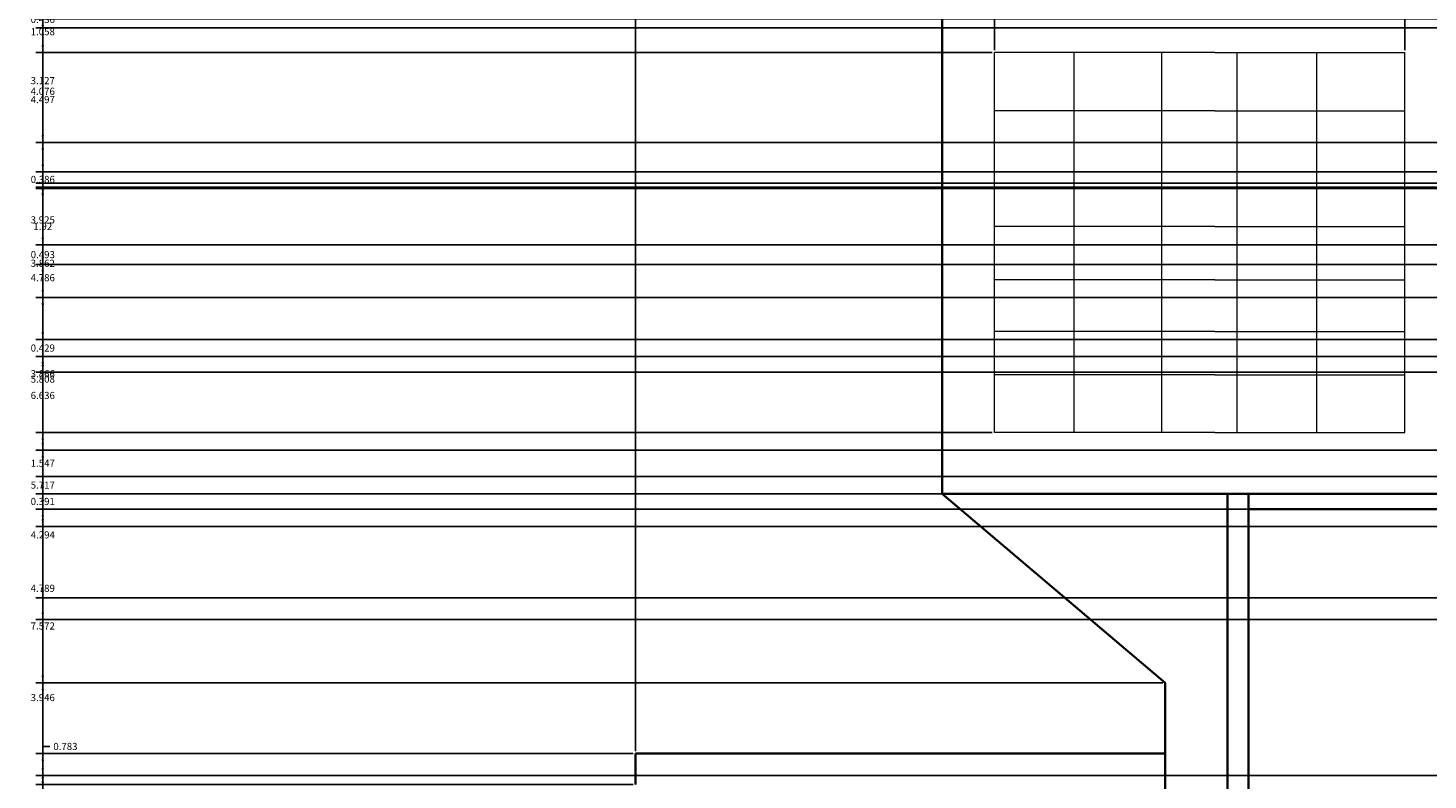
# Model space of a CAD drawing. Units: inches. Extents: x -10 to 130, y -32 to 34.
# Tile 2 of 22: x -10 to 26, y -13 to 6. Entities that reach past the tile are written whole.
import ezdxf

# ---------------------------------------------------------------- set-up
doc = ezdxf.new("R2010")
doc.units = ezdxf.units.IN
doc.header["$MEASUREMENT"] = 0
for name, color, linetype, lineweight in [('A-ANNO-DIMS', 2, 'Continuous', 18), ('A-ELEV', 7, 'Continuous', 35), ('A-GLAZ', 4, 'Continuous', 18)]:
    doc.layers.add(name, color=color, linetype=linetype, lineweight=lineweight)
doc.styles.get("Standard").update_dxf_attribs({"font": 'arial.ttf'})
doc.dimstyles.get("Standard").update_dxf_attribs({"dimtxt": 0.18, "dimasz": 0.18, "dimexe": 0.18, "dimexo": 0.0625, "dimgap": 0.09, "dimtad": 0, "dimtih": 1, "dimtoh": 1, "dimdec": 4, "dimzin": 0, "dimdsep": 46, "dimtxsty": 'Standard', "dimcen": 0.09, "dimadec": 0, "dimazin": 0, "dimtfac": 1, "dimtdec": 4, "dimtofl": 0, "dimtmove": 0, "dimatfit": 3, "dimfxl": 1, "dimtolj": 1, "dimtzin": 0, "dimarcsym": 0})

# ---------------------------------------------------------------- blocks, each defined once
blk = doc.blocks.new('*D11')
at = {"layer": 'A-ANNO-DIMS', "color": 0, "lineweight": -2, "transparency": 16777216}
for p, q in [((5.634, -12.739), (5.634, 33.879)), ((19.588, 19.547), (19.588, 33.879)), ((5.814, 33.699), (12.156, 33.699)), ((19.408, 33.699), (13.066, 33.699))]:
    blk.add_line(p, q, dxfattribs=at)
at = {"layer": 'A-ANNO-DIMS', "color": 0, "transparency": 16777216}
for points in [[(5.814, 33.729), (5.814, 33.669), (5.634, 33.699)], [(19.408, 33.729), (19.408, 33.669), (19.588, 33.699)]]:
    blk.add_solid(points, dxfattribs=at)
at = {"layer": 'Defpoints', "color": 0, "transparency": 16777216}
for p in [(19.588, 33.699), (19.588, 19.485), (5.634, -12.801)]:
    blk.add_point(p, dxfattribs=at)
at = {"layer": 'A-ANNO-DIMS', "color": 0, "transparency": 16777216, "insert": (12.611, 33.699), "char_height": 0.18, "attachment_point": 5}
blk.add_mtext('\\A1;13.954', dxfattribs=at)
blk = doc.blocks.new('*D30')
at = {"layer": 'A-ANNO-DIMS', "color": 0, "lineweight": -2, "transparency": 16777216}
for p, q in [((18.993, -11.011), (-9.564, -11.011)), ((-9.384, -11.191), (-9.384, -16.031)), ((-9.384, -21.234), (-9.384, -16.394)), ((8.226, -21.414), (-9.564, -21.414))]:
    blk.add_line(p, q, dxfattribs=at)
at = {"layer": 'A-ANNO-DIMS', "color": 0, "transparency": 16777216}
for points in [[(-9.414, -11.191), (-9.354, -11.191), (-9.384, -11.011)], [(-9.414, -21.234), (-9.354, -21.234), (-9.384, -21.414)]]:
    blk.add_solid(points, dxfattribs=at)
at = {"layer": 'Defpoints', "color": 0, "transparency": 16777216}
for p in [(-9.384, -11.011), (19.055, -11.011), (8.289, -21.414)]:
    blk.add_point(p, dxfattribs=at)
at = {"layer": 'A-ANNO-DIMS', "color": 0, "transparency": 16777216, "insert": (-9.384, -16.213), "char_height": 0.18, "attachment_point": 5}
blk.add_mtext('\\A1;10.404', dxfattribs=at)
blk = doc.blocks.new('*D31')
at = {"layer": 'A-ANNO-DIMS', "color": 0, "lineweight": -2, "transparency": 16777216}
for p, q in [((13.34, -6.222), (-9.564, -6.222)), ((-9.384, -6.402), (-9.384, -8.434)), ((-9.384, -10.831), (-9.384, -8.798)), ((18.993, -11.011), (-9.564, -11.011))]:
    blk.add_line(p, q, dxfattribs=at)
at = {"layer": 'A-ANNO-DIMS', "color": 0, "transparency": 16777216}
for points in [[(-9.414, -6.402), (-9.354, -6.402), (-9.384, -6.222)], [(-9.414, -10.831), (-9.354, -10.831), (-9.384, -11.011)]]:
    blk.add_solid(points, dxfattribs=at)
at = {"layer": 'Defpoints', "color": 0, "transparency": 16777216}
for p in [(-9.384, -6.222), (13.402, -6.222), (19.055, -11.011)]:
    blk.add_point(p, dxfattribs=at)
at = {"layer": 'A-ANNO-DIMS', "color": 0, "transparency": 16777216, "insert": (-9.384, -8.616), "char_height": 0.18, "attachment_point": 5}
blk.add_mtext('\\A1;4.789', dxfattribs=at)
blk = doc.blocks.new('*D32')
at = {"layer": 'A-ANNO-DIMS', "color": 0, "lineweight": -2, "transparency": 16777216}
for p, q in [((31.909, -0.414), (-9.564, -0.414)), ((-9.384, -0.594), (-9.384, -3.136)), ((-9.384, -6.042), (-9.384, -3.5)), ((13.34, -6.222), (-9.564, -6.222))]:
    blk.add_line(p, q, dxfattribs=at)
at = {"layer": 'A-ANNO-DIMS', "color": 0, "transparency": 16777216}
for points in [[(-9.414, -0.594), (-9.354, -0.594), (-9.384, -0.414)], [(-9.414, -6.042), (-9.354, -6.042), (-9.384, -6.222)]]:
    blk.add_solid(points, dxfattribs=at)
at = {"layer": 'Defpoints', "color": 0, "transparency": 16777216}
for p in [(-9.384, -0.414), (31.971, -0.414), (13.402, -6.222)]:
    blk.add_point(p, dxfattribs=at)
at = {"layer": 'A-ANNO-DIMS', "color": 0, "transparency": 16777216, "insert": (-9.384, -3.318), "char_height": 0.18, "attachment_point": 5}
blk.add_mtext('\\A1;5.808', dxfattribs=at)
blk = doc.blocks.new('*D33')
at = {"layer": 'A-ANNO-DIMS', "color": 0, "lineweight": -2, "transparency": 16777216}
for p, q in [((70.835, 1.511), (-9.564, 1.511)), ((-9.384, 1.331), (-9.384, 0.73)), ((-9.384, -0.234), (-9.384, 0.367)), ((31.909, -0.414), (-9.564, -0.414))]:
    blk.add_line(p, q, dxfattribs=at)
at = {"layer": 'A-ANNO-DIMS', "color": 0, "transparency": 16777216}
for points in [[(-9.414, 1.331), (-9.354, 1.331), (-9.384, 1.511)], [(-9.414, -0.234), (-9.354, -0.234), (-9.384, -0.414)]]:
    blk.add_solid(points, dxfattribs=at)
at = {"layer": 'Defpoints', "color": 0, "transparency": 16777216}
for p in [(-9.384, 1.511), (70.898, 1.511), (31.971, -0.414)]:
    blk.add_point(p, dxfattribs=at)
at = {"layer": 'A-ANNO-DIMS', "color": 0, "transparency": 16777216, "insert": (-9.384, 0.548), "char_height": 0.18, "attachment_point": 5}
blk.add_mtext('\\A1;1.92', dxfattribs=at)
blk = doc.blocks.new('*D34')
at = {"layer": 'A-ANNO-DIMS', "color": 0, "lineweight": -2, "transparency": 16777216}
for p, q in [((13.34, 6.007), (-9.564, 6.007)), ((-9.384, 5.827), (-9.384, 3.941)), ((-9.384, 1.691), (-9.384, 3.577)), ((70.835, 1.511), (-9.564, 1.511))]:
    blk.add_line(p, q, dxfattribs=at)
at = {"layer": 'A-ANNO-DIMS', "color": 0, "transparency": 16777216}
for points in [[(-9.414, 5.827), (-9.354, 5.827), (-9.384, 6.007)], [(-9.414, 1.691), (-9.354, 1.691), (-9.384, 1.511)]]:
    blk.add_solid(points, dxfattribs=at)
at = {"layer": 'Defpoints', "color": 0, "transparency": 16777216}
for p in [(-9.384, 6.007), (13.402, 6.007), (70.898, 1.511)]:
    blk.add_point(p, dxfattribs=at)
at = {"layer": 'A-ANNO-DIMS', "color": 0, "transparency": 16777216, "insert": (-9.384, 3.759), "char_height": 0.18, "attachment_point": 5}
blk.add_mtext('\\A1;4.497', dxfattribs=at)
blk = doc.blocks.new('*D46')
at = {"layer": 'A-ANNO-DIMS', "color": 0, "lineweight": -2, "transparency": 16777216}
for p, q in [((-9.384, -12.801), (-9.384, -12.621)), ((-9.384, -12.621), (-9.204, -12.621)), ((5.572, -12.801), (-9.564, -12.801)), ((-9.384, -13.404), (-9.384, -12.981)), ((5.572, -13.584), (-9.564, -13.584))]:
    blk.add_line(p, q, dxfattribs=at)
at = {"layer": 'A-ANNO-DIMS', "color": 0, "transparency": 16777216}
for points in [[(-9.414, -12.981), (-9.354, -12.981), (-9.384, -12.801)], [(-9.414, -13.404), (-9.354, -13.404), (-9.384, -13.584)]]:
    blk.add_solid(points, dxfattribs=at)
at = {"layer": 'Defpoints', "color": 0, "transparency": 16777216}
for p in [(-9.384, -12.801), (5.634, -12.801), (5.634, -13.584)]:
    blk.add_point(p, dxfattribs=at)
at = {"layer": 'A-ANNO-DIMS', "color": 0, "transparency": 16777216, "insert": (-8.81, -12.621), "char_height": 0.18, "attachment_point": 5}
blk.add_mtext('\\A1;0.783', dxfattribs=at)
blk = doc.blocks.new('*D49')
at = {"layer": 'A-ANNO-DIMS', "color": 0, "lineweight": -2, "transparency": 16777216}
for p, q in [((44.697, -13.356), (-9.564, -13.356)), ((-9.384, -13.536), (-9.384, -17.203)), ((-9.384, -21.234), (-9.384, -17.567)), ((44.697, -21.414), (-9.564, -21.414))]:
    blk.add_line(p, q, dxfattribs=at)
at = {"layer": 'A-ANNO-DIMS', "color": 0, "transparency": 16777216}
for points in [[(-9.414, -13.536), (-9.354, -13.536), (-9.384, -13.356)], [(-9.414, -21.234), (-9.354, -21.234), (-9.384, -21.414)]]:
    blk.add_solid(points, dxfattribs=at)
at = {"layer": 'Defpoints', "color": 0, "transparency": 16777216}
for p in [(44.76, -13.356), (-9.384, -21.414), (44.76, -21.414)]:
    blk.add_point(p, dxfattribs=at)
at = {"layer": 'A-ANNO-DIMS', "color": 0, "transparency": 16777216, "insert": (-9.384, -17.385), "char_height": 0.18, "attachment_point": 5}
blk.add_mtext('\\A1;8.059', dxfattribs=at)
blk = doc.blocks.new('*D90')
at = {"layer": 'A-ANNO-DIMS', "color": 0, "lineweight": -2, "transparency": 16777216}
for p, q in [((49.884, 5.802), (-9.564, 5.802)), ((-9.384, 5.622), (-9.384, 4.421)), ((-9.384, 2.855), (-9.384, 4.057)), ((49.884, 2.675), (-9.564, 2.675))]:
    blk.add_line(p, q, dxfattribs=at)
at = {"layer": 'A-ANNO-DIMS', "color": 0, "transparency": 16777216}
for points in [[(-9.414, 5.622), (-9.354, 5.622), (-9.384, 5.802)], [(-9.414, 2.855), (-9.354, 2.855), (-9.384, 2.675)]]:
    blk.add_solid(points, dxfattribs=at)
at = {"layer": 'Defpoints', "color": 0, "transparency": 16777216}
for p in [(49.946, 5.802), (-9.384, 2.675), (49.946, 2.675)]:
    blk.add_point(p, dxfattribs=at)
at = {"layer": 'A-ANNO-DIMS', "color": 0, "transparency": 16777216, "insert": (-9.384, 4.239), "char_height": 0.18, "attachment_point": 5}
blk.add_mtext('\\A1;3.127', dxfattribs=at)
blk = doc.blocks.new('*D91')
at = {"layer": 'A-ANNO-DIMS', "color": 0, "lineweight": -2, "transparency": 16777216}
for p, q in [((49.884, 2.675), (-9.564, 2.675)), ((-9.384, 2.495), (-9.384, 0.895)), ((-9.384, -1.07), (-9.384, 0.531)), ((49.884, -1.25), (-9.564, -1.25))]:
    blk.add_line(p, q, dxfattribs=at)
at = {"layer": 'A-ANNO-DIMS', "color": 0, "transparency": 16777216}
for points in [[(-9.414, 2.495), (-9.354, 2.495), (-9.384, 2.675)], [(-9.414, -1.07), (-9.354, -1.07), (-9.384, -1.25)]]:
    blk.add_solid(points, dxfattribs=at)
at = {"layer": 'Defpoints', "color": 0, "transparency": 16777216}
for p in [(49.946, 2.675), (-9.384, -1.25), (49.946, -1.25)]:
    blk.add_point(p, dxfattribs=at)
at = {"layer": 'A-ANNO-DIMS', "color": 0, "transparency": 16777216, "insert": (-9.384, 0.713), "char_height": 0.18, "attachment_point": 5}
blk.add_mtext('\\A1;3.925', dxfattribs=at)
blk = doc.blocks.new('*D92')
at = {"layer": 'A-ANNO-DIMS', "color": 0, "lineweight": -2, "transparency": 16777216}
for p, q in [((49.884, -1.25), (-9.564, -1.25)), ((-9.384, -1.43), (-9.384, -3.001)), ((-9.384, -4.936), (-9.384, -3.365)), ((49.884, -5.116), (-9.564, -5.116))]:
    blk.add_line(p, q, dxfattribs=at)
at = {"layer": 'A-ANNO-DIMS', "color": 0, "transparency": 16777216}
for points in [[(-9.414, -1.43), (-9.354, -1.43), (-9.384, -1.25)], [(-9.414, -4.936), (-9.354, -4.936), (-9.384, -5.116)]]:
    blk.add_solid(points, dxfattribs=at)
at = {"layer": 'Defpoints', "color": 0, "transparency": 16777216}
for p in [(49.946, -1.25), (-9.384, -5.116), (49.946, -5.116)]:
    blk.add_point(p, dxfattribs=at)
at = {"layer": 'A-ANNO-DIMS', "color": 0, "transparency": 16777216, "insert": (-9.384, -3.183), "char_height": 0.18, "attachment_point": 5}
blk.add_mtext('\\A1;3.866', dxfattribs=at)
blk = doc.blocks.new('*D93')
at = {"layer": 'A-ANNO-DIMS', "color": 0, "lineweight": -2, "transparency": 16777216}
for p, q in [((49.884, -5.116), (-9.564, -5.116)), ((-9.384, -5.296), (-9.384, -7.081)), ((-9.384, -9.23), (-9.384, -7.445)), ((49.884, -9.41), (-9.564, -9.41))]:
    blk.add_line(p, q, dxfattribs=at)
at = {"layer": 'A-ANNO-DIMS', "color": 0, "transparency": 16777216}
for points in [[(-9.414, -5.296), (-9.354, -5.296), (-9.384, -5.116)], [(-9.414, -9.23), (-9.354, -9.23), (-9.384, -9.41)]]:
    blk.add_solid(points, dxfattribs=at)
at = {"layer": 'Defpoints', "color": 0, "transparency": 16777216}
for p in [(49.946, -5.116), (-9.384, -9.41), (49.946, -9.41)]:
    blk.add_point(p, dxfattribs=at)
at = {"layer": 'A-ANNO-DIMS', "color": 0, "transparency": 16777216, "insert": (-9.384, -7.263), "char_height": 0.18, "attachment_point": 5}
blk.add_mtext('\\A1;4.294', dxfattribs=at)
blk = doc.blocks.new('*D94')
at = {"layer": 'A-ANNO-DIMS', "color": 0, "lineweight": -2, "transparency": 16777216}
for p, q in [((49.884, -9.41), (-9.564, -9.41)), ((-9.384, -9.59), (-9.384, -11.201)), ((-9.384, -13.176), (-9.384, -11.565)), ((49.884, -13.356), (-9.564, -13.356))]:
    blk.add_line(p, q, dxfattribs=at)
at = {"layer": 'A-ANNO-DIMS', "color": 0, "transparency": 16777216}
for points in [[(-9.414, -9.59), (-9.354, -9.59), (-9.384, -9.41)], [(-9.414, -13.176), (-9.354, -13.176), (-9.384, -13.356)]]:
    blk.add_solid(points, dxfattribs=at)
at = {"layer": 'Defpoints', "color": 0, "transparency": 16777216}
for p in [(49.946, -9.41), (-9.384, -13.356), (49.946, -13.356)]:
    blk.add_point(p, dxfattribs=at)
at = {"layer": 'A-ANNO-DIMS', "color": 0, "transparency": 16777216, "insert": (-9.384, -11.383), "char_height": 0.18, "attachment_point": 5}
blk.add_mtext('\\A1;3.946', dxfattribs=at)
blk = doc.blocks.new('*D111')
at = {"layer": 'A-ANNO-DIMS', "color": 0, "lineweight": -2, "transparency": 16777216}
for p, q in [((13.402, 6.07), (13.402, 33.879)), ((14.732, 5.012), (14.732, 33.879)), ((13.582, 33.699), (13.682, 33.699)), ((14.552, 33.699), (14.452, 33.699))]:
    blk.add_line(p, q, dxfattribs=at)
at = {"layer": 'A-ANNO-DIMS', "color": 0, "transparency": 16777216}
for points in [[(13.582, 33.729), (13.582, 33.669), (13.402, 33.699)], [(14.552, 33.729), (14.552, 33.669), (14.732, 33.699)]]:
    blk.add_solid(points, dxfattribs=at)
at = {"layer": 'Defpoints', "color": 0, "transparency": 16777216}
for p in [(14.732, 33.699), (13.402, 6.007), (14.732, 4.95)]:
    blk.add_point(p, dxfattribs=at)
at = {"layer": 'A-ANNO-DIMS', "color": 0, "transparency": 16777216, "insert": (14.067, 33.699), "char_height": 0.18, "attachment_point": 5}
blk.add_mtext('\\A1;1.330', dxfattribs=at)
blk = doc.blocks.new('*D112')
at = {"layer": 'A-ANNO-DIMS', "color": 0, "lineweight": -2, "transparency": 16777216}
for p, q in [((14.732, 5.012), (14.732, 33.879)), ((25.126, 5.012), (25.126, 33.879)), ((14.912, 33.699), (19.474, 33.699)), ((24.946, 33.699), (20.384, 33.699))]:
    blk.add_line(p, q, dxfattribs=at)
at = {"layer": 'A-ANNO-DIMS', "color": 0, "transparency": 16777216}
for points in [[(14.912, 33.729), (14.912, 33.669), (14.732, 33.699)], [(24.946, 33.729), (24.946, 33.669), (25.126, 33.699)]]:
    blk.add_solid(points, dxfattribs=at)
at = {"layer": 'Defpoints', "color": 0, "transparency": 16777216}
for p in [(25.126, 33.699), (14.732, 4.95), (25.126, 4.95)]:
    blk.add_point(p, dxfattribs=at)
at = {"layer": 'A-ANNO-DIMS', "color": 0, "transparency": 16777216, "insert": (19.929, 33.699), "char_height": 0.18, "attachment_point": 5}
blk.add_mtext('\\A1;10.394', dxfattribs=at)
blk = doc.blocks.new('*D113')
at = {"layer": 'A-ANNO-DIMS', "color": 0, "lineweight": -2, "transparency": 16777216}
for p, q in [((13.34, 6.007), (-9.564, 6.007)), ((-9.384, 5.827), (-9.384, 5.66)), ((-9.384, 5.13), (-9.384, 5.297)), ((14.67, 4.95), (-9.564, 4.95))]:
    blk.add_line(p, q, dxfattribs=at)
at = {"layer": 'A-ANNO-DIMS', "color": 0, "transparency": 16777216}
for points in [[(-9.414, 5.827), (-9.354, 5.827), (-9.384, 6.007)], [(-9.414, 5.13), (-9.354, 5.13), (-9.384, 4.95)]]:
    blk.add_solid(points, dxfattribs=at)
at = {"layer": 'Defpoints', "color": 0, "transparency": 16777216}
for p in [(-9.384, 6.007), (13.402, 6.007), (14.732, 4.95)]:
    blk.add_point(p, dxfattribs=at)
at = {"layer": 'A-ANNO-DIMS', "color": 0, "transparency": 16777216, "insert": (-9.384, 5.478), "char_height": 0.18, "attachment_point": 5}
blk.add_mtext('\\A1;1.058', dxfattribs=at)
blk = doc.blocks.new('*D114')
at = {"layer": 'A-ANNO-DIMS', "color": 0, "lineweight": -2, "transparency": 16777216}
for p, q in [((14.67, -4.675), (-9.564, -4.675)), ((-9.384, -4.855), (-9.384, -5.266)), ((-9.384, -6.042), (-9.384, -5.63)), ((13.34, -6.222), (-9.564, -6.222))]:
    blk.add_line(p, q, dxfattribs=at)
at = {"layer": 'A-ANNO-DIMS', "color": 0, "transparency": 16777216}
for points in [[(-9.414, -4.855), (-9.354, -4.855), (-9.384, -4.675)], [(-9.414, -6.042), (-9.354, -6.042), (-9.384, -6.222)]]:
    blk.add_solid(points, dxfattribs=at)
at = {"layer": 'Defpoints', "color": 0, "transparency": 16777216}
for p in [(14.732, -4.675), (-9.384, -6.222), (13.402, -6.222)]:
    blk.add_point(p, dxfattribs=at)
at = {"layer": 'A-ANNO-DIMS', "color": 0, "transparency": 16777216, "insert": (-9.384, -5.448), "char_height": 0.18, "attachment_point": 5}
blk.add_mtext('\\A1;1.547', dxfattribs=at)
blk = doc.blocks.new('*D115')
at = {"layer": 'A-ANNO-DIMS', "color": 0, "lineweight": -2, "transparency": 16777216}
for p, q in [((26.336, 6.007), (-9.564, 6.007)), ((-9.384, 5.827), (-9.384, 4.151)), ((-9.384, 2.111), (-9.384, 3.787)), ((26.336, 1.931), (-9.564, 1.931))]:
    blk.add_line(p, q, dxfattribs=at)
at = {"layer": 'A-ANNO-DIMS', "color": 0, "transparency": 16777216}
for points in [[(-9.414, 5.827), (-9.354, 5.827), (-9.384, 6.007)], [(-9.414, 2.111), (-9.354, 2.111), (-9.384, 1.931)]]:
    blk.add_solid(points, dxfattribs=at)
at = {"layer": 'Defpoints', "color": 0, "transparency": 16777216}
for p in [(26.399, 6.007), (-9.384, 1.931), (26.399, 1.931)]:
    blk.add_point(p, dxfattribs=at)
at = {"layer": 'A-ANNO-DIMS', "color": 0, "transparency": 16777216, "insert": (-9.384, 3.969), "char_height": 0.18, "attachment_point": 5}
blk.add_mtext('\\A1;4.076', dxfattribs=at)
blk = doc.blocks.new('*D116')
at = {"layer": 'A-ANNO-DIMS', "color": 0, "lineweight": -2, "transparency": 16777216}
for p, q in [((-9.383551, 2.111013), (-9.383551, 2.291013)), ((26.336278, 1.931013), (-9.563551, 1.931013)), ((26.336278, 1.544827), (-9.563551, 1.544827)), ((-9.383551, 1.364827), (-9.383551, 1.184827))]:
    blk.add_line(p, q, dxfattribs=at)
at = {"layer": 'A-ANNO-DIMS', "color": 0, "transparency": 16777216}
for points in [[(-9.413551, 2.111013), (-9.353551, 2.111013), (-9.383551, 1.931013)], [(-9.413551, 1.364827), (-9.353551, 1.364827), (-9.383551, 1.544827)]]:
    blk.add_solid(points, dxfattribs=at)
at = {"layer": 'Defpoints', "color": 0, "transparency": 16777216}
for p in [(26.398778, 1.931013), (-9.383551, 1.544827), (26.398778, 1.544827)]:
    blk.add_point(p, dxfattribs=at)
at = {"layer": 'A-ANNO-DIMS', "color": 0, "transparency": 16777216, "insert": (-9.383551, 1.73792), "char_height": 0.18, "attachment_point": 5}
blk.add_mtext('\\A1;0.386', dxfattribs=at)
blk = doc.blocks.new('*D117')
at = {"layer": 'A-ANNO-DIMS', "color": 0, "lineweight": -2, "transparency": 16777216}
for p, q in [((26.336, 1.545), (-9.564, 1.545)), ((-9.384, 1.365), (-9.384, -0.204)), ((-9.384, -2.137), (-9.384, -0.568)), ((26.336, -2.317), (-9.564, -2.317))]:
    blk.add_line(p, q, dxfattribs=at)
at = {"layer": 'A-ANNO-DIMS', "color": 0, "transparency": 16777216}
for points in [[(-9.414, 1.365), (-9.354, 1.365), (-9.384, 1.545)], [(-9.414, -2.137), (-9.354, -2.137), (-9.384, -2.317)]]:
    blk.add_solid(points, dxfattribs=at)
at = {"layer": 'Defpoints', "color": 0, "transparency": 16777216}
for p in [(26.399, 1.545), (-9.384, -2.317), (26.399, -2.317)]:
    blk.add_point(p, dxfattribs=at)
at = {"layer": 'A-ANNO-DIMS', "color": 0, "transparency": 16777216, "insert": (-9.384, -0.386), "char_height": 0.18, "attachment_point": 5}
blk.add_mtext('\\A1;3.862', dxfattribs=at)
blk = doc.blocks.new('*D118')
at = {"layer": 'A-ANNO-DIMS', "color": 0, "lineweight": -2, "transparency": 16777216}
for p, q in [((-9.384, -2.137), (-9.384, -1.957)), ((26.336, -2.317), (-9.564, -2.317)), ((26.336, -2.746), (-9.564, -2.746)), ((-9.384, -2.926), (-9.384, -3.106))]:
    blk.add_line(p, q, dxfattribs=at)
at = {"layer": 'A-ANNO-DIMS', "color": 0, "transparency": 16777216}
for points in [[(-9.414, -2.137), (-9.354, -2.137), (-9.384, -2.317)], [(-9.414, -2.926), (-9.354, -2.926), (-9.384, -2.746)]]:
    blk.add_solid(points, dxfattribs=at)
at = {"layer": 'Defpoints', "color": 0, "transparency": 16777216}
for p in [(26.399, -2.317), (-9.384, -2.746), (26.399, -2.746)]:
    blk.add_point(p, dxfattribs=at)
at = {"layer": 'A-ANNO-DIMS', "color": 0, "transparency": 16777216, "insert": (-9.384, -2.532), "char_height": 0.18, "attachment_point": 5}
blk.add_mtext('\\A1;0.429', dxfattribs=at)
blk = doc.blocks.new('*D121')
at = {"layer": 'A-ANNO-DIMS', "color": 0, "lineweight": -2, "transparency": 16777216}
for p, q in [((-9.384, 6.187), (-9.384, 6.367)), ((31.909, 6.007), (-9.564, 6.007)), ((32.427, 5.572), (-9.564, 5.572)), ((-9.384, 5.392), (-9.384, 5.212))]:
    blk.add_line(p, q, dxfattribs=at)
at = {"layer": 'A-ANNO-DIMS', "color": 0, "transparency": 16777216}
for points in [[(-9.414, 6.187), (-9.354, 6.187), (-9.384, 6.007)], [(-9.414, 5.392), (-9.354, 5.392), (-9.384, 5.572)]]:
    blk.add_solid(points, dxfattribs=at)
at = {"layer": 'Defpoints', "color": 0, "transparency": 16777216}
for p in [(-9.384, 6.007), (31.971, 6.007), (32.49, 5.572)]:
    blk.add_point(p, dxfattribs=at)
at = {"layer": 'A-ANNO-DIMS', "color": 0, "transparency": 16777216, "insert": (-9.384, 5.789), "char_height": 0.18, "attachment_point": 5}
blk.add_mtext('\\A1;0.436', dxfattribs=at)
blk = doc.blocks.new('*D122')
at = {"layer": 'A-ANNO-DIMS', "color": 0, "lineweight": -2, "transparency": 16777216}
for p, q in [((-9.383551, 0.25916), (-9.383551, 0.43916)), ((32.427309, 0.07916), (-9.563551, 0.07916)), ((31.908661, -0.413828), (-9.563551, -0.413828)), ((-9.383551, -0.593828), (-9.383551, -0.773828))]:
    blk.add_line(p, q, dxfattribs=at)
at = {"layer": 'A-ANNO-DIMS', "color": 0, "transparency": 16777216}
for points in [[(-9.413551, 0.25916), (-9.353551, 0.25916), (-9.383551, 0.07916)], [(-9.413551, -0.593828), (-9.353551, -0.593828), (-9.383551, -0.413828)]]:
    blk.add_solid(points, dxfattribs=at)
at = {"layer": 'Defpoints', "color": 0, "transparency": 16777216}
for p in [(32.489809, 0.07916), (-9.383551, -0.413828), (31.971161, -0.413828)]:
    blk.add_point(p, dxfattribs=at)
at = {"layer": 'A-ANNO-DIMS', "color": 0, "transparency": 16777216, "insert": (-9.383551, -0.167334), "char_height": 0.18, "attachment_point": 5}
blk.add_mtext('\\A1;0.493', dxfattribs=at)
blk = doc.blocks.new('*D125')
at = {"layer": 'A-ANNO-DIMS', "color": 0, "lineweight": -2, "transparency": 16777216}
for p, q in [((38.55, -0.414), (-9.564, -0.414)), ((-9.384, -0.594), (-9.384, -3.55)), ((-9.384, -6.87), (-9.384, -3.914)), ((38.55, -7.05), (-9.564, -7.05))]:
    blk.add_line(p, q, dxfattribs=at)
at = {"layer": 'A-ANNO-DIMS', "color": 0, "transparency": 16777216}
for points in [[(-9.414, -0.594), (-9.354, -0.594), (-9.384, -0.414)], [(-9.414, -6.87), (-9.354, -6.87), (-9.384, -7.05)]]:
    blk.add_solid(points, dxfattribs=at)
at = {"layer": 'Defpoints', "color": 0, "transparency": 16777216}
for p in [(38.612, -0.414), (-9.384, -7.05), (38.612, -7.05)]:
    blk.add_point(p, dxfattribs=at)
at = {"layer": 'A-ANNO-DIMS', "color": 0, "transparency": 16777216, "insert": (-9.384, -3.732), "char_height": 0.18, "attachment_point": 5}
blk.add_mtext('\\A1;6.636', dxfattribs=at)
blk = doc.blocks.new('*D127')
at = {"layer": 'A-ANNO-DIMS', "color": 0, "lineweight": -2, "transparency": 16777216}
for p, q in [((46.36, 1.642), (-9.564, 1.642)), ((-9.384, 1.462), (-9.384, -0.569)), ((-9.384, -2.964), (-9.384, -0.933)), ((46.36, -3.144), (-9.564, -3.144))]:
    blk.add_line(p, q, dxfattribs=at)
at = {"layer": 'A-ANNO-DIMS', "color": 0, "transparency": 16777216}
for points in [[(-9.414, 1.462), (-9.354, 1.462), (-9.384, 1.642)], [(-9.414, -2.964), (-9.354, -2.964), (-9.384, -3.144)]]:
    blk.add_solid(points, dxfattribs=at)
at = {"layer": 'Defpoints', "color": 0, "transparency": 16777216}
for p in [(46.423, 1.642), (-9.384, -3.144), (46.423, -3.144)]:
    blk.add_point(p, dxfattribs=at)
at = {"layer": 'A-ANNO-DIMS', "color": 0, "transparency": 16777216, "insert": (-9.384, -0.751), "char_height": 0.18, "attachment_point": 5}
blk.add_mtext('\\A1;4.786', dxfattribs=at)
blk = doc.blocks.new('*D129')
at = {"layer": 'A-ANNO-DIMS', "color": 0, "lineweight": -2, "transparency": 16777216}
for p, q in [((42.726, -3.144), (-9.564, -3.144)), ((-9.384, -3.324), (-9.384, -5.82)), ((-9.384, -8.681), (-9.384, -6.184)), ((42.726, -8.861), (-9.564, -8.861))]:
    blk.add_line(p, q, dxfattribs=at)
at = {"layer": 'A-ANNO-DIMS', "color": 0, "transparency": 16777216}
for points in [[(-9.414, -3.324), (-9.354, -3.324), (-9.384, -3.144)], [(-9.414, -8.681), (-9.354, -8.681), (-9.384, -8.861)]]:
    blk.add_solid(points, dxfattribs=at)
at = {"layer": 'Defpoints', "color": 0, "transparency": 16777216}
for p in [(42.788, -3.144), (-9.384, -8.861), (42.788, -8.861)]:
    blk.add_point(p, dxfattribs=at)
at = {"layer": 'A-ANNO-DIMS', "color": 0, "transparency": 16777216, "insert": (-9.384, -6.002), "char_height": 0.18, "attachment_point": 5}
blk.add_mtext('\\A1;5.717', dxfattribs=at)
blk = doc.blocks.new('*D130')
at = {"layer": 'A-ANNO-DIMS', "color": 0, "lineweight": -2, "transparency": 16777216}
for p, q in [((46.746, -5.784), (-9.564, -5.784)), ((-9.384, -5.964), (-9.384, -9.388)), ((-9.384, -13.176), (-9.384, -9.752)), ((46.746, -13.356), (-9.564, -13.356))]:
    blk.add_line(p, q, dxfattribs=at)
at = {"layer": 'A-ANNO-DIMS', "color": 0, "transparency": 16777216}
for points in [[(-9.414, -5.964), (-9.354, -5.964), (-9.384, -5.784)], [(-9.414, -13.176), (-9.354, -13.176), (-9.384, -13.356)]]:
    blk.add_solid(points, dxfattribs=at)
at = {"layer": 'Defpoints', "color": 0, "transparency": 16777216}
for p in [(46.809, -5.784), (-9.384, -13.356), (46.809, -13.356)]:
    blk.add_point(p, dxfattribs=at)
at = {"layer": 'A-ANNO-DIMS', "color": 0, "transparency": 16777216, "insert": (-9.384, -9.57), "char_height": 0.18, "attachment_point": 5}
blk.add_mtext('\\A1;7.572', dxfattribs=at)
blk = doc.blocks.new('*D131')
at = {"layer": 'A-ANNO-DIMS', "color": 0, "lineweight": -2, "transparency": 16777216}
for p, q in [((-9.384, -6.042), (-9.384, -5.862)), ((31.909, -6.222), (-9.564, -6.222)), ((31.909, -6.613), (-9.564, -6.613)), ((-9.384, -6.793), (-9.384, -6.973))]:
    blk.add_line(p, q, dxfattribs=at)
at = {"layer": 'A-ANNO-DIMS', "color": 0, "transparency": 16777216}
for points in [[(-9.414, -6.042), (-9.354, -6.042), (-9.384, -6.222)], [(-9.414, -6.793), (-9.354, -6.793), (-9.384, -6.613)]]:
    blk.add_solid(points, dxfattribs=at)
at = {"layer": 'Defpoints', "color": 0, "transparency": 16777216}
for p in [(31.971, -6.222), (-9.384, -6.613), (31.971, -6.613)]:
    blk.add_point(p, dxfattribs=at)
at = {"layer": 'A-ANNO-DIMS', "color": 0, "transparency": 16777216, "insert": (-9.384, -6.417), "char_height": 0.18, "attachment_point": 5}
blk.add_mtext('\\A1;0.391', dxfattribs=at)

msp = doc.modelspace()

# ---------------------------------------------------------------- linework, layer by layer
at = {"layer": 'A-ELEV'}
for p, q in [((13.4021, 6.0074), (13.4021, -6.2218)), ((13.4021, -6.2218), (26.3988, -6.2218)), ((13.4021, -6.2218), (19.055, -11.0106)), ((13.4021, -6.2218), (19.055, -11.0106)), ((20.6365, -6.2218), (20.6365, -16.1883)), ((21.1687, -6.2218), (21.1687, -16.1883)), ((21.1687, -6.6131), (26.3988, -6.6131)), ((19.055, -21.4145), (19.055, -11.0106)), ((19.055, -12.8012), (5.634, -12.8012)), ((5.634, -12.8012), (5.634, -13.5841))]:
    msp.add_line(p, q, dxfattribs=at)
at = {"layer": 'A-GLAZ'}
for p, q in [((19.5881, 4.9495), (14.7324, 4.9495)), ((14.7324, -4.6745), (14.7324, 4.9495)), ((16.7475, -4.6745), (16.7475, 4.9495)), ((18.9747, -4.6745), (18.9747, 4.9495)), ((20.3124, 4.9495), (19.5881, 4.9495)), ((20.3124, 4.9495), (25.1261, 4.9495)), ((20.8838, -4.6745), (20.8838, 4.9495)), ((22.8989, -4.6745), (22.8989, 4.9495)), ((25.1261, -4.6745), (25.1261, 4.9495)), ((19.5881, 3.4745), (14.7324, 3.4745)), ((20.3124, 3.4745), (19.5881, 3.4745)), ((20.3124, 3.4745), (25.1261, 3.4745)), ((19.5881, 1.9283), (14.7324, 1.9283)), ((20.3124, 1.9283), (19.5881, 1.9283)), ((20.3124, 1.9283), (25.1261, 1.9283)), ((19.5881, 0.5449), (14.7324, 0.5449)), ((20.3124, 0.5449), (19.5881, 0.5449)), ((20.3124, 0.5449), (25.1261, 0.5449)), ((19.5881, -0.809), (14.7324, -0.809)), ((20.3124, -0.809), (19.5881, -0.809)), ((20.3124, -0.809), (25.1261, -0.809)), ((19.5881, -2.111), (14.7324, -2.111)), ((20.3124, -2.111), (19.5881, -2.111)), ((20.3124, -2.111), (25.1261, -2.111)), ((19.5881, -3.2097), (14.7324, -3.2097)), ((20.3124, -3.2097), (19.5881, -3.2097)), ((20.3124, -3.2097), (25.1261, -3.2097)), ((19.5881, -4.6745), (14.7324, -4.6745)), ((20.3124, -4.6745), (19.5881, -4.6745)), ((20.3124, -4.6745), (25.1261, -4.6745))]:
    msp.add_line(p, q, dxfattribs=at)

# ---------------------------------------------------------------- dimensions: what is measured, and where the dimension line sits
at = {"layer": 'A-ANNO-DIMS'}
for base, p1, p2, picture, middle in [((19.5881, 33.6987), (5.634, -12.8012), (19.5881, 19.4845), '*D11', (12.611, 33.6987)), ((14.7324, 33.6987), (13.4021, 6.0074), (14.7324, 4.9495), '*D111', (14.0673, 33.6987)), ((25.1261, 33.6987), (14.7324, 4.9495), (25.1261, 4.9495), '*D112', (19.9293, 33.6987))]:
    dim = msp.add_linear_dim(base=base, p1=p1, p2=p2, dimstyle='Standard', override={"dimdec": 3, "dimlfac": 1, "dimrnd": 0, "dimzin": 0, "dimdsep": 46, "dimlunit": 2}, dxfattribs=at)
    dim.commit()
    dim.dimension.update_dxf_attribs({"geometry": picture, "text_midpoint": middle})
for base, p1, p2, override, picture, middle in [((-9.3836, 6.0074), (32.4898, 5.5715), (31.9712, 6.0074), {"dimdec": 3, "dimlfac": 1, "dimrnd": 0, "dimzin": 0, "dimdsep": 46, "dimlunit": 2}, '*D121', (-9.3836, 5.7895)), ((-9.3836, 6.0074), (70.898, 1.5107), (13.4021, 6.0074), {"dimdec": 3, "dimlfac": 1, "dimrnd": 0, "dimzin": 0, "dimdsep": 46, "dimlunit": 2}, '*D34', (-9.3836, 3.7591)), ((-9.3836, 6.0074), (14.7324, 4.9495), (13.4021, 6.0074), {"dimdec": 3, "dimlfac": 1, "dimrnd": 0, "dimzin": 0, "dimdsep": 46, "dimlunit": 2}, '*D113', (-9.3836, 5.4785)), ((-9.3836, 1.931), (26.3988, 6.0074), (26.3988, 1.931), {"dimdec": 3, "dimlfac": 1, "dimrnd": 0, "dimzin": 0, "dimdsep": 46, "dimlunit": 2}, '*D115', (-9.3836, 3.9692)), ((-9.3836, 2.6753), (49.9462, 5.8024), (49.9462, 2.6753), {"dimdec": 3, "dimlfac": 1, "dimrnd": 0, "dimzin": 0, "dimdsep": 46, "dimlunit": 2}, '*D90', (-9.3836, 4.2388)), ((-9.3836, -1.2496), (49.9462, 2.6753), (49.9462, -1.2496), {"dimdec": 3, "dimlfac": 1, "dimrnd": 0, "dimzin": 0, "dimdsep": 46, "dimlunit": 2}, '*D91', (-9.3836, 0.7128)), ((-9.3836, 1.5448), (26.3988, 1.931), (26.3988, 1.5448), {"dimdec": 3, "dimlfac": 1, "dimrnd": 0, "dimzin": 0, "dimdsep": 46, "dimlunit": 2}, '*D116', (-9.3836, 1.7379)), ((-9.3836, -3.1438), (46.4227, 1.6419), (46.4227, -3.1438), {"dimdec": 3, "dimlfac": 1, "dimrnd": 0, "dimzin": 0, "dimdsep": 46, "dimlunit": 2}, '*D127', (-9.3836, -0.751)), ((-9.3836, -2.317), (26.3988, 1.5448), (26.3988, -2.317), {"dimdec": 3, "dimlfac": 1, "dimrnd": 0, "dimzin": 0, "dimdsep": 46, "dimlunit": 2}, '*D117', (-9.3836, -0.3861)), ((-9.3836, 1.5107), (31.9712, -0.4138), (70.898, 1.5107), {"dimdec": 2, "dimlfac": 1, "dimrnd": 0, "dimzin": 0, "dimdsep": 46, "dimlunit": 2}, '*D33', (-9.3836, 0.5484)), ((-9.3836, -0.4138), (32.4898, 0.0792), (31.9712, -0.4138), {"dimdec": 3, "dimlfac": 1, "dimrnd": 0, "dimzin": 0, "dimdsep": 46, "dimlunit": 2}, '*D122', (-9.3836, -0.1673)), ((-9.3836, -0.4138), (13.4021, -6.2218), (31.9712, -0.4138), {"dimdec": 3, "dimlfac": 1, "dimrnd": 0, "dimzin": 0, "dimdsep": 46, "dimlunit": 2}, '*D32', (-9.3836, -3.3178)), ((-9.3836, -7.05), (38.6123, -0.4138), (38.6123, -7.05), {"dimdec": 3, "dimlfac": 1, "dimrnd": 0, "dimzin": 0, "dimdsep": 46, "dimlunit": 2}, '*D125', (-9.3836, -3.7319)), ((-9.3836, -5.1155), (49.9462, -1.2496), (49.9462, -5.1155), {"dimdec": 3, "dimlfac": 1, "dimrnd": 0, "dimzin": 0, "dimdsep": 46, "dimlunit": 2}, '*D92', (-9.3836, -3.1826)), ((-9.3836, -2.7461), (26.3988, -2.317), (26.3988, -2.7461), {"dimdec": 3, "dimlfac": 1, "dimrnd": 0, "dimzin": 0, "dimdsep": 46, "dimlunit": 2}, '*D118', (-9.3836, -2.5316)), ((-9.3836, -8.8608), (42.7881, -3.1438), (42.7881, -8.8608), {"dimdec": 3, "dimlfac": 1, "dimrnd": 0, "dimzin": 0, "dimdsep": 46, "dimlunit": 2}, '*D129', (-9.3836, -6.0023)), ((-9.3836, -6.2218), (14.7324, -4.6745), (13.4021, -6.2218), {"dimdec": 3, "dimlfac": 1, "dimrnd": 0, "dimzin": 0, "dimdsep": 46, "dimlunit": 2}, '*D114', (-9.3836, -5.4481)), ((-9.3836, -9.4098), (49.9462, -5.1155), (49.9462, -9.4098), {"dimdec": 3, "dimlfac": 1, "dimrnd": 0, "dimzin": 0, "dimdsep": 46, "dimlunit": 2}, '*D93', (-9.3836, -7.2626)), ((-9.3836, -13.3558), (46.8089, -5.7836), (46.8089, -13.3558), {"dimdec": 3, "dimlfac": 1, "dimrnd": 0, "dimzin": 0, "dimdsep": 46, "dimlunit": 2}, '*D130', (-9.3836, -9.5697)), ((-9.3836, -6.6131), (31.9712, -6.2218), (31.9712, -6.6131), {"dimdec": 3, "dimlfac": 1, "dimrnd": 0, "dimzin": 0, "dimdsep": 46, "dimlunit": 2}, '*D131', (-9.3836, -6.4175)), ((-9.3836, -6.2218), (19.055, -11.0106), (13.4021, -6.2218), {"dimdec": 3, "dimlfac": 1, "dimrnd": 0, "dimzin": 0, "dimdsep": 46, "dimlunit": 2}, '*D31', (-9.3836, -8.6162)), ((-9.3836, -13.3558), (49.9462, -9.4098), (49.9462, -13.3558), {"dimdec": 3, "dimlfac": 1, "dimrnd": 0, "dimzin": 0, "dimdsep": 46, "dimlunit": 2}, '*D94', (-9.3836, -11.3828)), ((-9.3836, -11.0106), (8.2886, -21.4145), (19.055, -11.0106), {"dimdec": 3, "dimlfac": 1, "dimrnd": 0, "dimzin": 0, "dimdsep": 46, "dimlunit": 2}, '*D30', (-9.3836, -16.2125)), ((-9.3836, -12.8012), (5.634, -13.5841), (5.634, -12.8012), {"dimdec": 3, "dimlfac": 1, "dimrnd": 0, "dimzin": 0, "dimdsep": 46, "dimlunit": 2}, '*D46', (-8.8098, -12.6212)), ((-9.3836, -21.4145), (44.76, -13.3558), (44.76, -21.4145), {"dimdec": 3, "dimlfac": 1, "dimrnd": 0, "dimzin": 0, "dimdsep": 46, "dimlunit": 2}, '*D49', (-9.3836, -17.3852))]:
    dim = msp.add_linear_dim(base=base, p1=p1, p2=p2, angle=90, dimstyle='Standard', override=override, dxfattribs=at)
    dim.commit()
    dim.dimension.update_dxf_attribs({"geometry": picture, "text_midpoint": middle})

doc.saveas('drawing.dxf')
